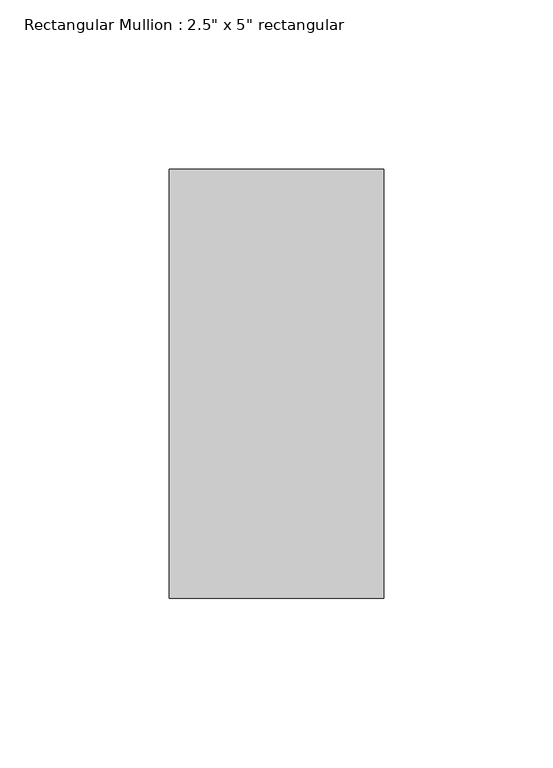
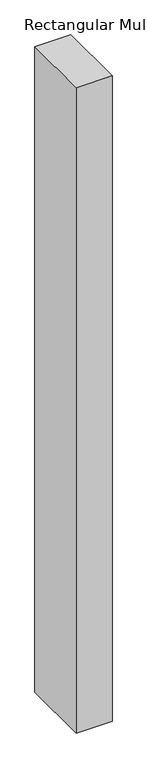
"""IFC4 building model written with IfcOpenShell, lengths in millimetres: member geometry."""

from ifc_helpers import new_model, si_unit, frame, origin, place, context, project, spatial, polyline, outline, extrude, source, transform, mapped, element, save


def member_77473497(model_context):
    return source(origin(), model_context, "Body", "SweptSolid", [
        extrude(outline(polyline([(0.0, 63.5), (0.0, -63.5), (-63.5, -63.5), (-63.5, 63.5), (0.0, 63.5)])), frame((0.0, 0.0, -1209.3898707), z_axis=(0.0, 0.0, 1.0), x_axis=(1.0, 0.0, 0.0)), (0.0, 0.0, 1.0), 1209.3898707),
    ])


if __name__ == "__main__":
    model = new_model("IFC4")
    model_context = context("Model", 3, world=origin())
    ifc_project = project(units=[si_unit("LENGTHUNIT", "METRE", prefix="MILLI")], contexts=[model_context])
    site = spatial("IfcSite", under=ifc_project)
    building = spatial("IfcBuilding", under=site)
    placement = place(None, origin())
    member_shape = member_77473497(model_context)
    element("IfcMember", 1, ObjectType="Rectangular Mullion : 2.5\" x 5\" rectangular", at=placement, inside=building, context=model_context, shape_type="MappedRepresentation", body=[
        mapped(member_shape, transform((0.0, 0.0, 0.0), x_axis=(1.0, 0.0, 0.0), y_axis=(0.0, 1.0, 0.0), z_axis=(0.0, 0.0, 1.0))),
    ])
    save(model, "model.ifc")

# Revit data of these elements
# Type "Rectangular Mullion : 2.5\" x 5\" rectangular"
#   built-in parameter 1007304 = 0.416667 (stored number, unit not read)
#   built-in parameter 1007301 = 0.104167 (stored number, unit not read)
#   built-in parameter 1007300 = 0.104167 (stored number, unit not read)
# Element 1 (IfcMember, "Rectangular Mullion : 2.5\" x 5\" rectangular")
#   Materials on its faces: "Aluminum"
# Materials
#   "Aluminum": class "Metal", colour RGB 247 247 247, transparency 0, Description = "Aluminum 6061", Cost = 0
